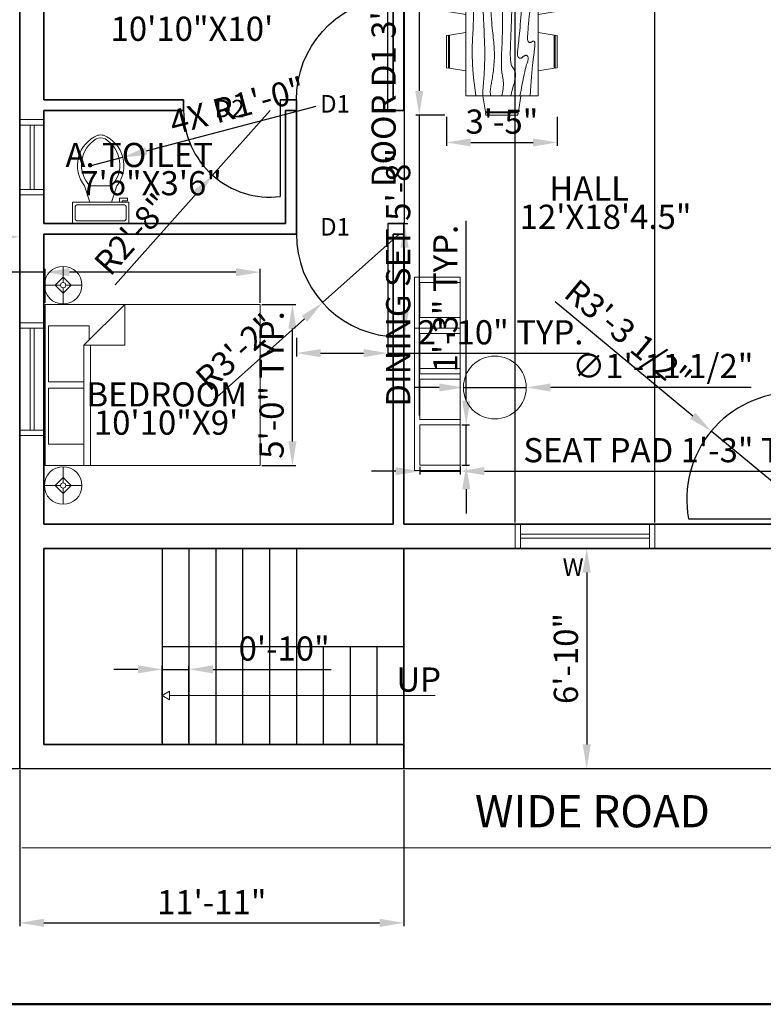
# Model space of a CAD drawing. Units: inches. Extents: x 2113 to 4530, y 1685 to 2353.
# Tile 2 of 6: x 2314 to 2591, y 1685 to 2052. Entities that reach past the tile are written whole.
import ezdxf

# ---------------------------------------------------------------- set-up
doc = ezdxf.new("R2010")
doc.units = ezdxf.units.IN
for name, color, linetype, lineweight in [('A-ANNO-DIMS', 2, 'Continuous', 18), ('A-ANNO-SYMB', 7, 'Continuous', 18), ('A-ANNO-TEXT', 7, 'Continuous', 18), ('A-ANNO-TTLB', 7, 'Continuous', 50), ('A-AREA-IDEN', 7, 'Continuous', 18), ('A-DOOR', 3, 'Continuous', 25), ('A-FLOR-FIXT', 9, 'Continuous', 18), ('A-FLOR-STRS', 7, 'Continuous', 25), ('A-FURN', 8, 'Continuous', 18), ('A-GLAZ', 4, 'Continuous', 18), ('A-WALL', 7, 'Continuous', 35), ('C-PROP', 7, 'Continuous', 25), ('C-ROAD', 8, 'Continuous', 18), ('S-ANNO-DIMS', 2, 'Continuous', 18)]:
    doc.layers.add(name, color=color, linetype=linetype, lineweight=lineweight)
doc.styles.get("Standard").update_dxf_attribs({"font": 'arial.ttf'})
doc.dimstyles.new('ISO-25', dxfattribs={"dimtxt": 9, "dimasz": 9, "dimexe": 1.25, "dimexo": 0.625, "dimgap": 2, "dimtad": 1, "dimdec": 1, "dimlunit": 4, "dimtxsty": 'Standard', "dimcen": 2.5, "dimazin": 0, "dimtfac": 1, "dimtdec": 1, "dimtmove": 0, "dimatfit": 3, "dimfxl": 1, "dimarcsym": 0})

# ---------------------------------------------------------------- blocks, each defined once
blk = doc.blocks.new('Toilet - top')
for p, q in [((9.5, -6), (9.5, -2)), ((-10, -8.5), (-8, -8.5)), ((-10, -9.5), (-10, -8.5)), ((-7, -9.5), (-10, -9.5)), ((-8, -8.5), (-8, -8)), ((-7, -8), (-7, -9.5)), ((-4, -8), (-6, -14)), ((4, -8), (6, -14)), ((4, -14), (-4, -14))]:
    blk.add_line(p, q)
blk.add_lwpolyline([(10.5, -8), (10.5, 0), (-10.5, 0), (-10.5, -8)], close=True)
for points in [[(-9.5, -2), (-9.5, -6)], [(8.5, -1), (-8.5, -1)], [(-8.5, -7), (8.5, -7)]]:
    blk.add_lwpolyline(points)
for centre, radius, start, end in [((-8.62, -1.88), 0.884, 81.8699, 188.1301), ((8.62, -1.88), 0.884, 351.8699, 98.1301), ((-8.62, -6.12), 0.884, 171.8699, 278.1301), ((8.62, -6.12), 0.884, 261.8699, 8.1301), ((3.52, -21.58), 12.17, 141.4691, 247.9714), ((4.2, -21.82), 11.33, 136.3677, 238.9468), ((-3.52, -21.58), 12.17, 292.0284, 38.5307), ((-4.2, -21.82), 11.33, 301.053, 43.6321), ((0, -27.88), 4, 245.7318, 294.2682), ((0, -29), 4, 254.8605, 285.1395)]:
    blk.add_arc(centre, radius, start, end)
blk = doc.blocks.new('Dining Set - 36 x 72 in.')
for p, q in [((-22.2343, 26.00059), (-23.4847, 17.99762)), ((-22.2304, 26), (-5.7608, 26)), ((-22, 27.5), (-22.1562, 26.50042)), ((-5.8416, 26.5), (-22.1534, 26.5)), ((-22, 27.5), (-6, 27.5)), ((-5.8437, 26.49966), (-6, 27.5)), ((-4.5152, 17.99762), (-5.7655, 25.99926)), ((5.7657, 26.00059), (4.5153, 17.99762)), ((5.7696, 26), (22.2392, 26)), ((6, 27.5), (5.8438, 26.50042)), ((22.1584, 26.5), (5.8466, 26.5)), ((6, 27.5), (22, 27.5)), ((22.1563, 26.49966), (22, 27.5)), ((23.4848, 17.99762), (22.2345, 25.99926)), ((36, 18), (-36, 18)), ((-36, 18), (-36, -18)), ((36, -18), (36, 18)), ((-45.5, 8), (-44.5004, 8.15617)), ((-45.5, 8), (-45.5, -8)), ((-44.5, -8.15843), (-44.5, 8.15338)), ((-44.0006, 8.23428), (-35.9976, 9.48474)), ((-44, 8.23041), (-44, -8.23915)), ((44.0006, 8.23428), (35.9976, 9.48474)), ((44, 8.23041), (44, -8.23915)), ((44.5, -8.15843), (44.5, 8.15338)), ((45.5, 8), (44.5005, 8.15617)), ((45.5, 8), (45.5, -8)), ((-44.4997, -8.15631), (-45.5, -8)), ((-35.9976, -9.48476), (-43.9993, -8.2345)), ((35.9976, -9.48476), (43.9993, -8.2345)), ((44.4997, -8.15631), (45.5, -8)), ((-36, -18), (36, -18)), ((-22.2343, -26.0006), (-23.4847, -17.99762)), ((-4.5152, -17.99762), (-5.7655, -25.99928)), ((5.7657, -26.0006), (4.5153, -17.99762)), ((23.4848, -17.99762), (22.2345, -25.99928)), ((-22.2304, -26), (-5.7608, -26)), ((-22, -27.5), (-22.1562, -26.50044)), ((-5.8416, -26.5), (-22.1534, -26.5)), ((-22, -27.5), (-6, -27.5)), ((-5.8437, -26.49967), (-6, -27.5)), ((5.7696, -26), (22.2392, -26)), ((6, -27.5), (5.8438, -26.50044)), ((22.1584, -26.5), (5.8466, -26.5)), ((6, -27.5), (22, -27.5)), ((22.1563, -26.49967), (22, -27.5))]:
    blk.add_line(p, q)
for points in [[(-36, 15), (-31.1772, 14.97754), (-26.8079, 14.91406), (-22.8538, 14.81543), (-19.276, 14.6875), (-16.0362, 14.53613), (-13.0957, 14.36718), (-10.4159, 14.18652), (-7.9583, 14), (-5.6904, 13.81315), (-3.6035, 13.63021), (-1.6954, 13.45508), (0.0365, 13.29166), (1.5945, 13.14388), (2.9811, 13.01562), (4.1988, 12.9108), (5.25, 12.83333), (6.1393, 12.78613), (6.8802, 12.76823), (7.4883, 12.77767), (7.9792, 12.8125), (8.3685, 12.87077), (8.6719, 12.95052), (8.9049, 13.0498), (9.0833, 13.16666), (9.2205, 13.29899), (9.3216, 13.44401), (9.3895, 13.59879), (9.4271, 13.76041), (9.4373, 13.92594), (9.4232, 14.09245), (9.3875, 14.257), (9.3333, 14.41666), (9.2638, 14.56917), (9.1836, 14.71484), (9.0975, 14.85465), (9.0104, 14.98958), (8.9272, 15.1206), (8.8529, 15.2487), (8.7922, 15.37483), (8.75, 15.5), (8.7305, 15.62467), (8.7344, 15.74739), (8.7617, 15.86621), (8.8125, 15.97916), (8.8867, 16.08431), (8.9844, 16.17968), (9.1055, 16.26334), (9.25, 16.33333), (9.4189, 16.38802), (9.6172, 16.42708), (9.8506, 16.45052), (10.125, 16.45833), (10.4463, 16.45052), (10.8203, 16.42708), (11.2529, 16.38802), (11.75, 16.33333), (12.3184, 16.26318), (12.9694, 16.17838), (13.7151, 16.07991), (14.5677, 15.96875), (15.5395, 15.84586), (16.6426, 15.71224), (17.8893, 15.56884), (19.2917, 15.41666), (20.859, 15.25667), (22.5879, 15.08984), (24.4721, 14.91715), (26.5052, 14.73958), (28.6809, 14.5581), (30.9929, 14.3737), (33.4347, 14.18733), (36, 14)], [(-36, 10), (-28.9766, 10.14274), (-23.1725, 10.20442), (-18.4241, 10.19775), (-14.5677, 10.13541), (-11.4399, 10.03011), (-8.877, 9.89453), (-6.7154, 9.74137), (-4.7917, 9.58333), (-2.9698, 9.43082), (-1.2246, 9.28515), (0.4415, 9.14534), (2.026, 9.01041), (3.5266, 8.87939), (4.9408, 8.7513), (6.266, 8.62516), (7.5, 8.5), (8.6411, 8.37549), (9.6914, 8.2539), (10.6538, 8.13818), (11.5312, 8.03125), (12.3267, 7.93603), (13.043, 7.85547), (13.6831, 7.79248), (14.25, 7.75), (14.7471, 7.7303), (15.1797, 7.73307), (15.5537, 7.75732), (15.875, 7.80208), (16.1494, 7.86637), (16.3828, 7.94922), (16.5811, 8.04964), (16.75, 8.16666), (16.8944, 8.29915), (17.0143, 8.44531), (17.1089, 8.60319), (17.1771, 8.77083), (17.218, 8.94629), (17.2305, 9.1276), (17.2137, 9.31282), (17.1667, 9.5), (17.0895, 9.6875), (16.987, 9.875), (16.8649, 10.0625), (16.7292, 10.25), (16.5856, 10.4375), (16.4401, 10.625), (16.2985, 10.8125), (16.1667, 11), (16.05, 11.18733), (15.9518, 11.3737), (15.8752, 11.5581), (15.8229, 11.73958), (15.798, 11.91715), (15.8034, 12.08984), (15.842, 12.25667), (15.9167, 12.41666), (16.0295, 12.56836), (16.1784, 12.70833), (16.3605, 12.83268), (16.5729, 12.9375), (16.8127, 13.01888), (17.0768, 13.07291), (17.3625, 13.0957), (17.6667, 13.08333), (17.9894, 13.03312), (18.3418, 12.94726), (18.7382, 12.82918), (19.1927, 12.68229), (19.7195, 12.51001), (20.3327, 12.31575), (21.0465, 12.10294), (21.875, 11.875), (22.8357, 11.63354), (23.959, 11.37304), (25.2786, 11.08618), (26.8282, 10.76562), (28.6414, 10.40405), (30.752, 9.99414), (33.1936, 9.52856), (36, 9)], [(-36, 5.5), (-30.7157, 5.3348), (-26.069, 5.20963), (-21.9946, 5.11767), (-18.4271, 5.05208), (-15.3009, 5.00602), (-12.5508, 4.97265), (-10.1112, 4.94515), (-7.9167, 4.91666), (-5.909, 4.88167), (-4.0586, 4.83984), (-2.3429, 4.79215), (-0.7396, 4.73958), (0.7739, 4.6831), (2.22, 4.6237), (3.6213, 4.56233), (5, 4.5), (6.373, 4.43782), (7.7344, 4.3776), (9.0723, 4.32129), (10.375, 4.27083), (11.6309, 4.22819), (12.8281, 4.19531), (13.9551, 4.17415), (15, 4.16666), (15.954, 4.17448), (16.819, 4.19791), (17.6001, 4.23698), (18.3021, 4.29166), (18.9299, 4.36198), (19.4883, 4.44791), (19.9823, 4.54948), (20.4167, 4.66666), (20.7969, 4.79899), (21.1302, 4.94401), (21.4245, 5.09879), (21.6875, 5.26041), (21.9271, 5.42594), (22.1511, 5.59245), (22.3672, 5.757), (22.5834, 5.91666), (22.8065, 6.06868), (23.0404, 6.21093), (23.2879, 6.34147), (23.5521, 6.45833), (23.8358, 6.55957), (24.142, 6.64323), (24.4735, 6.70735), (24.8334, 6.75), (25.2235, 6.76969), (25.642, 6.76692), (26.0858, 6.74267), (26.5521, 6.69791), (27.0379, 6.63362), (27.5404, 6.55078), (28.0565, 6.45036), (28.5834, 6.33333), (29.1242, 6.19987), (29.7071, 6.04687), (30.3661, 5.87044), (31.1354, 5.66666), (32.0493, 5.43164), (33.142, 5.16146), (34.4475, 4.85221), (36, 4.5)], [(-36, -1), (-30.7915, -0.6591), (-26.0195, -0.38216), (-21.6519, -0.16284), (-17.6563, 0.00521), (-14.0005, 0.12833), (-10.6523, 0.21289), (-7.5796, 0.26522), (-4.75, 0.29166), (-2.134, 0.29793), (0.2878, 0.28711), (2.5317, 0.26163), (4.6146, 0.22396), (6.5529, 0.17651), (8.3633, 0.12174), (10.0623, 0.06209), (11.6667, 0), (13.1899, -0.06201), (14.6341, -0.1211), (15.9982, -0.17432), (17.2813, -0.21875), (18.4823, -0.25147), (19.6003, -0.26953), (20.6343, -0.27002), (21.5834, -0.25), (22.4481, -0.20768), (23.2357, -0.14584), (23.9549, -0.06836), (24.6146, 0.02083), (25.2235, 0.11784), (25.7904, 0.21875), (26.3241, 0.31966), (26.8334, 0.41666), (27.3265, 0.50618), (27.8099, 0.58593), (28.2894, 0.65397), (28.7709, 0.70833), (29.2601, 0.74707), (29.763, 0.76823), (30.2855, 0.76985), (30.8334, 0.75), (31.4088, 0.70784), (31.9994, 0.64713), (32.589, 0.57275), (33.1615, 0.48958), (33.7008, 0.4025), (34.1908, 0.3164), (34.6153, 0.23616), (34.9584, 0.16666), (35.2099, 0.11165), (35.3848, 0.07031), (35.504, 0.04069), (35.5886, 0.02083), (35.6594, 0.00879), (35.7377, 0.0026), (35.8442, 0.00032), (36, 0)], [(-36, -6.5), (-27.1843, -6.31267), (-20.084, -6.1263), (-14.469, -5.9419), (-10.1094, -5.76042), (-6.7752, -5.58285), (-4.2363, -5.41016), (-2.2629, -5.24333), (-0.625, -5.08334), (0.8708, -4.93099), (2.2715, -4.78646), (3.5872, -4.64974), (4.8281, -4.52084), (6.0046, -4.39974), (7.127, -4.28646), (8.2053, -4.18099), (9.25, -4.08334), (10.2705, -3.99382), (11.2734, -3.91407), (12.2647, -3.84603), (13.25, -3.79167), (14.2354, -3.75293), (15.2266, -3.73177), (16.2295, -3.73015), (17.25, -3.75), (18.2912, -3.79248), (19.3451, -3.85547), (20.4009, -3.93604), (21.4479, -4.03125), (22.4754, -4.13819), (23.4727, -4.25391), (24.4289, -4.37549), (25.3334, -4.5), (26.1785, -4.62492), (26.9694, -4.74935), (27.7145, -4.87281), (28.4219, -4.99479), (29.1, -5.11483), (29.7572, -5.23242), (30.4016, -5.34709), (31.0417, -5.45834), (31.6837, -5.56437), (32.3262, -5.65821), (32.9658, -5.73153), (33.599, -5.77604), (34.2224, -5.78345), (34.8327, -5.74545), (35.4264, -5.65373), (36, -5.5)], [(-36, -10), (-26.4022, -9.81299), (-18.4675, -9.62891), (-11.9839, -9.45069), (-6.7396, -9.28125), (-2.5226, -9.12354), (0.8789, -8.98047), (3.6769, -8.85498), (6.0833, -8.75), (8.2767, -8.66765), (10.3021, -8.60677), (12.1712, -8.56543), (13.8958, -8.54167), (15.4876, -8.53353), (16.9583, -8.53907), (18.3197, -8.55632), (19.5834, -8.58334), (20.7616, -8.61841), (21.8685, -8.66081), (22.9188, -8.71004), (23.9271, -8.76563), (24.9081, -8.82707), (25.8763, -8.89388), (26.8465, -8.96558), (27.8334, -9.04167), (28.8474, -9.12118), (29.8828, -9.20117), (30.93, -9.27824), (31.9792, -9.34896), (33.0205, -9.40991), (34.0443, -9.45768), (35.0407, -9.48885), (36, -9.5)], [(-36, -14.5), (-30.0881, -14.33513), (-25.0332, -14.21224), (-20.7312, -14.12647), (-17.0781, -14.07292), (-13.97, -14.04671), (-11.3027, -14.04297), (-8.9724, -14.05681), (-6.875, -14.08334), (-4.9224, -14.11833), (-3.0905, -14.16016), (-1.3709, -14.20785), (0.2448, -14.26042), (1.7647, -14.3169), (3.1973, -14.3763), (4.5507, -14.43767), (5.8333, -14.5), (7.0554, -14.5621), (8.235, -14.62175), (9.3922, -14.67652), (10.5469, -14.72396), (11.7192, -14.76164), (12.929, -14.78711), (14.1965, -14.79794), (15.5417, -14.79167), (16.9933, -14.76424), (18.6152, -14.70508), (20.4804, -14.60197), (22.6615, -14.44271), (25.2312, -14.21509), (28.2624, -13.9069), (31.8277, -13.50594), (36, -13)]]:
    blk.add_lwpolyline(points)
blk = doc.blocks.new('Bed - Queen')
for p, q in [((0, -80.00003), (0, 0)), ((0, 0), (59.99999, 0)), ((59.99999, 0), (59.99999, -80.00003)), ((7.99999, -1.2), (28.79998, -1.2)), ((7.99999, -14.4), (7.99999, -1.2)), ((28.79998, -1.2), (28.79998, -14.4)), ((31.19999, -1.2), (51.99999, -1.2)), ((31.19999, -14.4), (31.19999, -1.2)), ((51.99999, -1.2), (51.99999, -16.4)), ((0, -14.4), (44.8, -14.4)), ((59.99999, -29.6), (44.8, -14.4)), ((44.8, -14.4), (44.8, -29.6)), ((44.8, -16.8), (0, -16.8)), ((51.99999, -16.4), (46.79936, -16.4)), ((44.8, -29.6), (59.99999, -29.6)), ((59.99999, -80.00003), (0, -80.00003))]:
    blk.add_line(p, q)
blk = doc.blocks.new('Lamp - Table')
for p, q in [((0, 7), (0, 1)), ((-1, 0), (-7, 0)), ((0, 3), (-3, 0)), ((-3, 0), (0, -3)), ((3, 0), (0, 3)), ((0, -3), (3, 0)), ((1, 0), (7, 0)), ((0, -1), (0, -7))]:
    blk.add_line(p, q)
for radius in [7, 1]:
    blk.add_circle((0, 0), radius)
blk = doc.blocks.new('*D26')
at = {"layer": 'A-ANNO-DIMS', "color": 0, "lineweight": -2, "transparency": 16777216}
for p, q in [((2457.36, 1854.89), (2526.08, 1854.89)), ((2524.83, 1845.89), (2524.83, 1781.89)), ((2457.36, 1772.89), (2526.08, 1772.89))]:
    blk.add_line(p, q, dxfattribs=at)
at = {"layer": 'A-ANNO-DIMS', "color": 0, "transparency": 16777216}
for points in [[(2523.33, 1845.89), (2526.33, 1845.89), (2524.83, 1854.89)], [(2523.33, 1781.89), (2526.33, 1781.89), (2524.83, 1772.89)]]:
    blk.add_solid(points, dxfattribs=at)
at = {"layer": 'Defpoints', "color": 0, "transparency": 16777216}
for p in [(2456.73, 1854.89), (2456.73, 1772.89), (2524.83, 1772.89)]:
    blk.add_point(p, dxfattribs=at)
at = {"layer": 'A-ANNO-DIMS', "color": 0, "transparency": 16777216, "insert": (2518.23, 1813.89), "char_height": 9, "attachment_point": 5, "rotation": 90}
blk.add_mtext('6\'-10"', dxfattribs=at)
blk = doc.blocks.new('*D29')
at = {"layer": 'A-ANNO-DIMS', "color": 0, "lineweight": -2, "transparency": 16777216}
for p, q in [((2289.73, 2168.26), (2289.73, 1969.64)), ((2313.73, 2150.26), (2313.73, 1969.64)), ((2304.73, 1970.89), (2298.73, 1970.89))]:
    blk.add_line(p, q, dxfattribs=at)
at = {"layer": 'A-ANNO-DIMS', "color": 0, "transparency": 16777216}
for points in [[(2298.73, 1972.39), (2298.73, 1969.39), (2289.73, 1970.89)], [(2304.73, 1972.39), (2304.73, 1969.39), (2313.73, 1970.89)]]:
    blk.add_solid(points, dxfattribs=at)
at = {"layer": 'Defpoints', "color": 0, "transparency": 16777216}
for p in [(2289.73, 2168.89), (2313.73, 2150.89), (2289.73, 1970.89)]:
    blk.add_point(p, dxfattribs=at)
at = {"layer": 'A-ANNO-DIMS', "color": 0, "transparency": 16777216, "insert": (2301.73, 1977.4), "char_height": 9, "attachment_point": 5}
blk.add_mtext("2'", dxfattribs=at)
blk = doc.blocks.new('DOOR-D1-SWING')
blk.add_line((34, 42), (34, 0))
blk.add_arc((38.24, 38), 38.24, 180, 263.6403)
blk = doc.blocks.new('SOFA-SEAT-PAD')
for p, q in [((0, 15), (0, 0)), ((0, 15), (15, 15)), ((0, 0), (15, 0))]:
    blk.add_line(p, q)
blk = doc.blocks.new('LOT-465X396')
blk.add_line((0, 0), (465, 0))
blk = doc.blocks.new('*D40')
at = {"layer": 'Defpoints', "color": 0, "transparency": 16777216}
for p in [(2323.25, 1957.72), (2323.25, 1945.72), (2403.25, 1945.72)]:
    blk.add_point(p, dxfattribs=at)
at = {"layer": 'S-ANNO-DIMS', "color": 0, "lineweight": -2, "transparency": 16777216}
for p, q in [((2323.25, 1946.35), (2323.25, 1958.97)), ((2403.25, 1946.35), (2403.25, 1958.97)), ((2323.25, 1957.72), (2177.86, 1957.72)), ((2394.25, 1957.72), (2332.25, 1957.72))]:
    blk.add_line(p, q, dxfattribs=at)
at = {"layer": 'S-ANNO-DIMS', "color": 0, "transparency": 16777216}
for points in [[(2332.25, 1959.22), (2332.25, 1956.22), (2323.25, 1957.72)], [(2394.25, 1959.22), (2394.25, 1956.22), (2403.25, 1957.72)]]:
    blk.add_solid(points, dxfattribs=at)
at = {"layer": 'S-ANNO-DIMS', "color": 0, "transparency": 16777216, "insert": (2246.05, 1964.65), "char_height": 9, "attachment_point": 5}
blk.add_mtext('QUEEN BED 6\'-8" TYP.', dxfattribs=at)
blk = doc.blocks.new('*D41')
at = {"layer": 'Defpoints', "color": 0, "transparency": 16777216}
for p in [(2403.25, 1945.72), (2415.25, 1945.72), (2403.25, 1885.72)]:
    blk.add_point(p, dxfattribs=at)
at = {"layer": 'S-ANNO-DIMS', "color": 0, "lineweight": -2, "transparency": 16777216}
for p, q in [((2403.87, 1945.72), (2416.5, 1945.72)), ((2415.25, 1894.72), (2415.25, 1936.72)), ((2403.87, 1885.72), (2416.5, 1885.72))]:
    blk.add_line(p, q, dxfattribs=at)
at = {"layer": 'S-ANNO-DIMS', "color": 0, "transparency": 16777216}
for points in [[(2413.75, 1936.72), (2416.75, 1936.72), (2415.25, 1945.72)], [(2413.75, 1894.72), (2416.75, 1894.72), (2415.25, 1885.72)]]:
    blk.add_solid(points, dxfattribs=at)
at = {"layer": 'S-ANNO-DIMS', "color": 0, "transparency": 16777216, "insert": (2408.65, 1915.72), "char_height": 9, "attachment_point": 5, "rotation": 90}
blk.add_mtext('5\'-0" TYP.', dxfattribs=at)
blk = doc.blocks.new('*D50')
at = {"layer": 'Defpoints', "color": 0, "transparency": 16777216}
for p in [(2462.73, 1885.89), (2477.73, 1885.89), (2477.73, 1883.64)]:
    blk.add_point(p, dxfattribs=at)
at = {"layer": 'S-ANNO-DIMS', "color": 0, "lineweight": -2, "transparency": 16777216}
for p, q in [((2462.73, 1885.26), (2462.73, 1882.39)), ((2477.73, 1885.26), (2477.73, 1882.39)), ((2453.73, 1883.64), (2444.73, 1883.64)), ((2462.73, 1883.64), (2477.73, 1883.64)), ((2486.73, 1883.64), (2620.23, 1883.64))]:
    blk.add_line(p, q, dxfattribs=at)
at = {"layer": 'S-ANNO-DIMS', "color": 0, "transparency": 16777216}
for points in [[(2453.73, 1885.14), (2453.73, 1882.14), (2462.73, 1883.64)], [(2486.73, 1885.14), (2486.73, 1882.14), (2477.73, 1883.64)]]:
    blk.add_solid(points, dxfattribs=at)
at = {"layer": 'S-ANNO-DIMS', "color": 0, "transparency": 16777216, "insert": (2557.98, 1890.29), "char_height": 9, "attachment_point": 5}
blk.add_mtext('SEAT PAD 1\'-3" TYP.', dxfattribs=at)
blk = doc.blocks.new('*D51')
at = {"layer": 'Defpoints', "color": 0, "transparency": 16777216}
for p in [(2477.73, 1900.89), (2479.98, 1900.89), (2477.73, 1885.89)]:
    blk.add_point(p, dxfattribs=at)
at = {"layer": 'S-ANNO-DIMS', "color": 0, "lineweight": -2, "transparency": 16777216}
for p, q in [((2479.98, 1909.89), (2479.98, 1976.9)), ((2478.36, 1900.89), (2481.23, 1900.89)), ((2479.98, 1885.89), (2479.98, 1900.89)), ((2478.36, 1885.89), (2481.23, 1885.89)), ((2479.98, 1876.89), (2479.98, 1867.89))]:
    blk.add_line(p, q, dxfattribs=at)
at = {"layer": 'S-ANNO-DIMS', "color": 0, "transparency": 16777216}
for points in [[(2478.48, 1909.89), (2481.48, 1909.89), (2479.98, 1900.89)], [(2478.48, 1876.89), (2481.48, 1876.89), (2479.98, 1885.89)]]:
    blk.add_solid(points, dxfattribs=at)
at = {"layer": 'S-ANNO-DIMS', "color": 0, "transparency": 16777216, "insert": (2473.38, 1947.89), "char_height": 9, "attachment_point": 5, "rotation": 90}
blk.add_mtext('1\'-3" TYP.', dxfattribs=at)
blk = doc.blocks.new('*D54')
at = {"layer": 'Defpoints', "color": 0, "transparency": 16777216}
for p in [(2450.73, 1975.89), (2457.03, 1975.89), (2450.73, 1933.89)]:
    blk.add_point(p, dxfattribs=at)
at = {"layer": 'S-ANNO-DIMS', "color": 0, "lineweight": -2, "transparency": 16777216}
for p, q in [((2457.03, 1975.89), (2457.03, 2104.07)), ((2451.36, 1975.89), (2458.28, 1975.89)), ((2457.03, 1942.89), (2457.03, 1966.89)), ((2451.36, 1933.89), (2458.28, 1933.89))]:
    blk.add_line(p, q, dxfattribs=at)
at = {"layer": 'S-ANNO-DIMS', "color": 0, "transparency": 16777216}
for points in [[(2455.53, 1966.89), (2458.53, 1966.89), (2457.03, 1975.89)], [(2455.53, 1942.89), (2458.53, 1942.89), (2457.03, 1933.89)]]:
    blk.add_solid(points, dxfattribs=at)
at = {"layer": 'S-ANNO-DIMS', "color": 0, "transparency": 16777216, "insert": (2450.37, 2044.48), "char_height": 9, "attachment_point": 5, "rotation": 90}
blk.add_mtext('DOOR D1 3\'-6" TYP.', dxfattribs=at)
blk = doc.blocks.new('*D55')
at = {"layer": 'Defpoints', "color": 0, "transparency": 16777216}
for p in [(2416.73, 1933.89), (2450.73, 1933.89), (2450.73, 1927.59)]:
    blk.add_point(p, dxfattribs=at)
at = {"layer": 'S-ANNO-DIMS', "color": 0, "lineweight": -2, "transparency": 16777216}
for p, q in [((2416.73, 1933.26), (2416.73, 1926.34)), ((2450.73, 1933.26), (2450.73, 1926.34)), ((2425.73, 1927.59), (2441.73, 1927.59)), ((2450.73, 1927.59), (2525.74, 1927.59))]:
    blk.add_line(p, q, dxfattribs=at)
at = {"layer": 'S-ANNO-DIMS', "color": 0, "transparency": 16777216}
for points in [[(2425.73, 1929.09), (2425.73, 1926.09), (2416.73, 1927.59)], [(2441.73, 1929.09), (2441.73, 1926.09), (2450.73, 1927.59)]]:
    blk.add_solid(points, dxfattribs=at)
at = {"layer": 'S-ANNO-DIMS', "color": 0, "transparency": 16777216, "insert": (2492.74, 1934.18), "char_height": 9, "attachment_point": 5}
blk.add_mtext('2\'-10" TYP.', dxfattribs=at)
blk = doc.blocks.new('*D58')
at = {"layer": 'Defpoints', "color": 0, "transparency": 16777216}
for p in [(2472.67, 2084.34), (2462.46, 2016.25), (2472.67, 2016.25)]:
    blk.add_point(p, dxfattribs=at)
at = {"layer": 'S-ANNO-DIMS', "color": 0, "lineweight": -2, "transparency": 16777216}
for p, q in [((2472.05, 2084.34), (2461.21, 2084.34)), ((2462.46, 2075.34), (2462.46, 2025.25)), ((2472.05, 2016.25), (2461.21, 2016.25)), ((2462.46, 2016.25), (2462.46, 1904.33))]:
    blk.add_line(p, q, dxfattribs=at)
at = {"layer": 'S-ANNO-DIMS', "color": 0, "transparency": 16777216}
for points in [[(2460.96, 2075.34), (2463.96, 2075.34), (2462.46, 2084.34)], [(2460.96, 2025.25), (2463.96, 2025.25), (2462.46, 2016.25)]]:
    blk.add_solid(points, dxfattribs=at)
at = {"layer": 'S-ANNO-DIMS', "color": 0, "transparency": 16777216, "insert": (2455.81, 1955.79), "char_height": 9, "attachment_point": 5, "rotation": 90}
blk.add_mtext('DINING SET 5\'-8"', dxfattribs=at)
blk = doc.blocks.new('*D59')
at = {"layer": 'Defpoints', "color": 0, "transparency": 16777216}
for p in [(2472.67, 2016.25), (2513.83, 2016.25), (2513.83, 2006.03)]:
    blk.add_point(p, dxfattribs=at)
at = {"layer": 'S-ANNO-DIMS', "color": 0, "lineweight": -2, "transparency": 16777216}
for p, q in [((2472.67, 2015.62), (2472.67, 2004.78)), ((2513.83, 2015.62), (2513.83, 2004.78)), ((2481.67, 2006.03), (2504.83, 2006.03))]:
    blk.add_line(p, q, dxfattribs=at)
at = {"layer": 'S-ANNO-DIMS', "color": 0, "transparency": 16777216}
for points in [[(2481.67, 2007.53), (2481.67, 2004.53), (2472.67, 2006.03)], [(2504.83, 2007.53), (2504.83, 2004.53), (2513.83, 2006.03)]]:
    blk.add_solid(points, dxfattribs=at)
at = {"layer": 'S-ANNO-DIMS', "color": 0, "transparency": 16777216, "insert": (2493.25, 2012.63), "char_height": 9, "attachment_point": 5}
blk.add_mtext('3\'-5"', dxfattribs=at)
blk = doc.blocks.new('*D90')
at = {"layer": 'Defpoints', "color": 0, "transparency": 16777216}
for p in [(2313.73, 1772.89), (2456.73, 1772.89), (2456.73, 1715.45)]:
    blk.add_point(p, dxfattribs=at)
at = {"layer": 'S-ANNO-DIMS', "color": 0, "lineweight": -2, "transparency": 16777216}
for p, q in [((2313.73, 1772.26), (2313.73, 1714.2)), ((2456.73, 1772.26), (2456.73, 1714.2)), ((2322.73, 1715.45), (2447.73, 1715.45))]:
    blk.add_line(p, q, dxfattribs=at)
at = {"layer": 'S-ANNO-DIMS', "color": 0, "transparency": 16777216}
for points in [[(2322.73, 1716.95), (2322.73, 1713.95), (2313.73, 1715.45)], [(2447.73, 1716.95), (2447.73, 1713.95), (2456.73, 1715.45)]]:
    blk.add_solid(points, dxfattribs=at)
at = {"layer": 'S-ANNO-DIMS', "color": 0, "transparency": 16777216, "insert": (2385.23, 1721.97), "char_height": 9, "attachment_point": 5}
blk.add_mtext('11\'-11"', dxfattribs=at)
blk = doc.blocks.new('*D93')
at = {"layer": 'Defpoints', "color": 0, "transparency": 16777216}
for p in [(2550.184017, 2196.835797), (2498.184017, 1863.885797), (2550.184017, 1863.885797)]:
    blk.add_point(p, dxfattribs=at)
at = {"layer": 'S-ANNO-DIMS', "color": 0, "lineweight": -2, "transparency": 16777216}
for p, q in [((2498.184017, 1864.510797), (2498.184017, 2198.085797)), ((2507.184017, 2196.835797), (2541.184017, 2196.835797)), ((2550.184017, 1864.510797), (2550.184017, 2198.085797))]:
    blk.add_line(p, q, dxfattribs=at)
at = {"layer": 'S-ANNO-DIMS', "color": 0, "transparency": 16777216}
for points in [[(2507.184017, 2198.335797), (2507.184017, 2195.335797), (2498.184017, 2196.835797)], [(2541.184017, 2198.335797), (2541.184017, 2195.335797), (2550.184017, 2196.835797)]]:
    blk.add_solid(points, dxfattribs=at)
at = {"layer": 'S-ANNO-DIMS', "color": 0, "transparency": 16777216, "insert": (2524.184017, 2203.335797), "char_height": 9, "attachment_point": 5}
blk.add_mtext('4\'-4"', dxfattribs=at)
blk = doc.blocks.new('*D94')
at = {"layer": 'Defpoints', "color": 0, "transparency": 16777216}
for p in [(2376.73, 1809.84), (2366.73, 1781.89), (2376.73, 1781.89)]:
    blk.add_point(p, dxfattribs=at)
at = {"layer": 'S-ANNO-DIMS', "color": 0, "lineweight": -2, "transparency": 16777216}
for p, q in [((2357.73, 1809.84), (2348.73, 1809.84)), ((2366.73, 1782.51), (2366.73, 1811.09)), ((2366.73, 1809.84), (2376.73, 1809.84)), ((2376.73, 1782.51), (2376.73, 1811.09)), ((2385.73, 1809.84), (2429.65, 1809.84))]:
    blk.add_line(p, q, dxfattribs=at)
at = {"layer": 'S-ANNO-DIMS', "color": 0, "transparency": 16777216}
for points in [[(2357.73, 1811.34), (2357.73, 1808.34), (2366.73, 1809.84)], [(2385.73, 1811.34), (2385.73, 1808.34), (2376.73, 1809.84)]]:
    blk.add_solid(points, dxfattribs=at)
at = {"layer": 'S-ANNO-DIMS', "color": 0, "transparency": 16777216, "insert": (2412.19, 1816.43), "char_height": 9, "attachment_point": 5}
blk.add_mtext('0\'-10"', dxfattribs=at)
blk = doc.blocks.new('*D102')
at = {"layer": 'Defpoints', "color": 0, "transparency": 16777216}
for p in [(2571.2, 1898.54), (2601.73, 1873.2)]:
    blk.add_point(p, dxfattribs=at)
at = {"layer": 'S-ANNO-DIMS', "color": 0, "lineweight": -2, "transparency": 16777216}
for p, q in [((2513.09, 1946.76), (2564.27, 1904.29)), ((2601.73, 1873.2), (2571.2, 1898.54))]:
    blk.add_line(p, q, dxfattribs=at)
at = {"layer": 'S-ANNO-DIMS', "color": 0, "transparency": 16777216}
blk.add_solid([(2565.23, 1905.45), (2563.31, 1903.14), (2571.2, 1898.54)], dxfattribs=at)
at = {"layer": 'S-ANNO-DIMS', "color": 0, "transparency": 16777216, "insert": (2539.47, 1933.52), "char_height": 9, "attachment_point": 5, "rotation": 320.315}
blk.add_mtext('R3\'-3 1/2"', dxfattribs=at)
blk = doc.blocks.new('*D104')
at = {"layer": 'Defpoints', "color": 0, "transparency": 16777216}
for p in [(2454.97, 1971.89), (2426.47, 1946.39)]:
    blk.add_point(p, dxfattribs=at)
at = {"layer": 'S-ANNO-DIMS', "color": 0, "lineweight": -2, "transparency": 16777216}
for p, q in [((2454.97, 1971.89), (2426.47, 1946.39)), ((2385.83, 1910.03), (2419.77, 1940.39))]:
    blk.add_line(p, q, dxfattribs=at)
at = {"layer": 'S-ANNO-DIMS', "color": 0, "transparency": 16777216}
blk.add_solid([(2418.77, 1941.51), (2420.77, 1939.27), (2426.47, 1946.39)], dxfattribs=at)
at = {"layer": 'S-ANNO-DIMS', "color": 0, "transparency": 16777216, "insert": (2395.04, 1927.12), "char_height": 9, "attachment_point": 5, "rotation": 41.8197}
blk.add_mtext('R3\'-2"', dxfattribs=at)
blk = doc.blocks.new('*D106')
at = {"layer": 'Defpoints', "color": 0, "transparency": 16777216}
for p in [(2406.95, 2017.89), (2385.55, 1993.8)]:
    blk.add_point(p, dxfattribs=at)
at = {"layer": 'S-ANNO-DIMS', "color": 0, "lineweight": -2, "transparency": 16777216}
for p, q in [((2406.95, 2017.89), (2385.55, 1993.8)), ((2349.31, 1953.04), (2379.57, 1987.08))]:
    blk.add_line(p, q, dxfattribs=at)
at = {"layer": 'S-ANNO-DIMS', "color": 0, "transparency": 16777216}
blk.add_solid([(2378.45, 1988.07), (2380.69, 1986.08), (2385.55, 1993.8)], dxfattribs=at)
at = {"layer": 'S-ANNO-DIMS', "color": 0, "transparency": 16777216, "insert": (2356.52, 1971.08), "char_height": 9, "attachment_point": 5, "rotation": 48.3656}
blk.add_mtext('R2\'-8"', dxfattribs=at)
blk = doc.blocks.new('*D107')
at = {"layer": 'Defpoints', "color": 0, "transparency": 16777216}
for p in [(2478.94, 1914.79), (2502.33, 1914.79)]:
    blk.add_point(p, dxfattribs=at)
at = {"layer": 'S-ANNO-DIMS', "color": 0, "lineweight": -2, "transparency": 16777216}
for p, q in [((2469.94, 1914.79), (2460.94, 1914.79)), ((2478.94, 1914.79), (2502.33, 1914.79)), ((2586.01, 1914.78), (2511.33, 1914.78))]:
    blk.add_line(p, q, dxfattribs=at)
at = {"layer": 'S-ANNO-DIMS', "color": 0, "transparency": 16777216}
for points in [[(2469.94, 1916.29), (2469.94, 1913.29), (2478.94, 1914.79)], [(2511.33, 1916.28), (2511.33, 1913.28), (2502.33, 1914.79)]]:
    blk.add_solid(points, dxfattribs=at)
at = {"layer": 'S-ANNO-DIMS', "color": 0, "transparency": 16777216, "insert": (2553.17, 1921.63), "char_height": 9, "attachment_point": 5, "rotation": 359.9989}
blk.add_mtext('∅1\'-11 1/2"', dxfattribs=at)
blk = doc.blocks.new('*D108')
at = {"layer": 'Defpoints', "color": 0, "transparency": 16777216}
for p in [(2352.13, 2000.5), (2340.36, 1997.41)]:
    blk.add_point(p, dxfattribs=at)
at = {"layer": 'S-ANNO-DIMS', "color": 0, "lineweight": -2, "transparency": 16777216}
for p, q in [((2423.93, 2019.36), (2360.84, 2002.79)), ((2340.36, 1997.41), (2352.13, 2000.5))]:
    blk.add_line(p, q, dxfattribs=at)
at = {"layer": 'S-ANNO-DIMS', "color": 0, "transparency": 16777216}
blk.add_solid([(2360.45, 2004.24), (2361.22, 2001.34), (2352.13, 2000.5)], dxfattribs=at)
at = {"layer": 'S-ANNO-DIMS', "color": 0, "transparency": 16777216, "insert": (2395.06, 2018.6), "char_height": 9, "attachment_point": 5, "rotation": 14.7198}
blk.add_mtext('4X R1\'-0"', dxfattribs=at)

msp = doc.modelspace()

# ---------------------------------------------------------------- linework, layer by layer
at = {"layer": 'A-ANNO-SYMB'}
for p, q in [((2366.73, 1800.14), (2369.51, 1801.73)), ((2366.73, 1800.14), (2369.51, 1798.54)), ((2369.51, 1801.73), (2369.51, 1798.54)), ((2369.51, 1800.14), (2468.39, 1800.14))]:
    msp.add_line(p, q, dxfattribs=at)
at = {"layer": 'A-ANNO-TTLB'}
msp.add_lwpolyline([(2112.77, 2352.97), (4498.42, 2352.97), (4498.42, 1685.12), (2112.77, 1685.12)], close=True, dxfattribs=at)
at = {"layer": 'A-DOOR'}
for p, q in [((2410.73, 2021.89), (2410.73, 1985.89)), ((2562.73, 1865.89), (2610.73, 1865.89))]:
    msp.add_line(p, q, dxfattribs=at)
for centre, radius, start, end in [((2406.95, 2017.89), 32.22, 180, 276.7329), ((2601.73, 1873.2), 39.68, 90, 190.6291)]:
    msp.add_arc(centre, radius, start, end, dxfattribs=at)
at = {"layer": 'A-FLOR-STRS'}
for p, q in [((2366.73, 1854.89), (2366.73, 1781.89)), ((2376.73, 1854.89), (2376.73, 1781.89)), ((2386.73, 1854.89), (2386.73, 1781.89)), ((2396.73, 1854.89), (2396.73, 1781.89)), ((2406.73, 1854.89), (2406.73, 1781.89)), ((2416.73, 1854.89), (2416.73, 1781.89)), ((2366.73, 1818.39), (2456.73, 1818.39)), ((2426.73, 1818.39), (2426.73, 1781.89)), ((2436.73, 1818.39), (2436.73, 1781.89)), ((2446.73, 1818.39), (2446.73, 1781.89))]:
    msp.add_line(p, q, dxfattribs=at)
at = {"layer": 'A-FURN'}
for p, q in [((2460.73, 1955.89), (2460.73, 1883.89)), ((2460.73, 1955.89), (2477.73, 1955.89)), ((2477.73, 1955.89), (2477.73, 1883.89)), ((2462.73, 1953.89), (2477.73, 1953.89)), ((2462.73, 1953.89), (2462.73, 1940.89)), ((2462.73, 1940.89), (2477.73, 1940.89)), ((2460.73, 1936.89), (2477.73, 1936.89)), ((2462.73, 1921.89), (2477.73, 1921.89)), ((2460.73, 1883.89), (2477.73, 1883.89))]:
    msp.add_line(p, q, dxfattribs=at)
msp.add_circle((2490.63, 1914.79), 11.69, dxfattribs=at)
at = {"layer": 'A-GLAZ'}
for p, q in [((2322.73, 2014.53), (2313.73, 2014.53)), ((2322.73, 2012.53), (2313.73, 2012.53)), ((2317.67, 1988.53), (2317.67, 2012.53)), ((2319.17, 1988.53), (2319.17, 2012.53)), ((2322.73, 1988.53), (2313.73, 1988.53)), ((2322.73, 1986.53), (2313.73, 1986.53)), ((2313.73, 1938.89), (2322.73, 1938.89)), ((2313.73, 1936.89), (2322.73, 1936.89)), ((2317.67, 1898.89), (2317.67, 1936.89)), ((2319.17, 1898.89), (2319.17, 1936.89)), ((2313.73, 1898.89), (2322.73, 1898.89)), ((2313.73, 1896.89), (2322.73, 1896.89)), ((2498.18, 1863.89), (2498.18, 1854.89)), ((2500.18, 1863.89), (2500.18, 1854.89)), ((2548.18, 1863.89), (2548.18, 1854.89)), ((2550.18, 1863.89), (2550.18, 1854.89)), ((2500.18, 1860.14), (2548.18, 1860.14)), ((2500.18, 1858.64), (2548.18, 1858.64))]:
    msp.add_line(p, q, dxfattribs=at)
at = {"layer": 'A-WALL'}
for p, q in [((2313.73, 2150.89), (2313.73, 1772.89)), ((2322.73, 2141.89), (2322.73, 2021.89)), ((2452.73, 2141.89), (2452.73, 2021.89)), ((2456.73, 2089.89), (2456.73, 2017.89)), ((2322.73, 2021.89), (2374.73, 2021.89)), ((2322.73, 2021.89), (2374.73, 2021.89)), ((2374.73, 2021.89), (2374.73, 2017.89)), ((2410.73, 2021.89), (2416.73, 2021.89)), ((2410.73, 2021.89), (2416.73, 2021.89)), ((2416.73, 2021.89), (2416.73, 1971.89)), ((2450.73, 2021.89), (2452.73, 2021.89)), ((2322.73, 2017.89), (2374.73, 2017.89)), ((2322.73, 2017.89), (2374.73, 2017.89)), ((2322.73, 2017.89), (2322.73, 1975.89)), ((2412.73, 2017.89), (2412.73, 1975.89)), ((2412.73, 2017.89), (2416.73, 2017.89)), ((2450.73, 2017.89), (2456.73, 2017.89)), ((2452.73, 2017.89), (2456.73, 2017.89)), ((2322.73, 1975.89), (2412.73, 1975.89)), ((2450.73, 1975.89), (2456.73, 1975.89)), ((2456.73, 1975.89), (2456.73, 1863.89)), ((2322.73, 1971.89), (2416.73, 1971.89)), ((2322.73, 1971.89), (2322.73, 1863.89)), ((2452.73, 1971.89), (2452.73, 1863.89)), ((2452.73, 1971.89), (2456.73, 1971.89)), ((2322.73, 1863.89), (2452.73, 1863.89)), ((2456.73, 1863.89), (2610.73, 1863.89)), ((2322.73, 1854.89), (2650.73, 1854.89)), ((2322.73, 1854.89), (2322.73, 1781.89)), ((2456.73, 1854.89), (2456.73, 1772.89)), ((2322.73, 1781.89), (2456.73, 1781.89))]:
    msp.add_line(p, q, dxfattribs=at)
at = {"layer": 'C-ROAD'}
msp.add_line((2314.56, 1743.4), (2754.73, 1743.4), dxfattribs=at)

# ---------------------------------------------------------------- block references
at = {"layer": 'A-DOOR', "extrusion": (0, 0, -1), "zscale": -1, "rotation": 180}
msp.add_blockref('DOOR-D1-SWING', (-2416.73, 2059.89), dxfattribs=at)
at = {"layer": 'A-DOOR'}
msp.add_blockref('DOOR-D1-SWING', (2416.73, 1933.89), dxfattribs=at)
at = {"layer": 'A-FLOR-FIXT', "rotation": 180}
msp.add_blockref('Toilet - top', (2343.88, 1975.83), dxfattribs=at)
at = {"layer": 'A-FURN', "xscale": 0.7483003964013882, "yscale": 0.7483003964013882, "zscale": 0.7483003964013882, "rotation": 269.9999999999999}
msp.add_blockref('Dining Set - 36 x 72 in.', (2493.25, 2050.3), dxfattribs=at)
at = {"layer": 'A-FURN'}
for name, p, rotation in [('Lamp - Table', (2329.91, 1952.9), 180), ('Bed - Queen', (2323.25, 1885.72), 90), ('Lamp - Table', (2329.91, 1878.29), 180)]:
    msp.add_blockref(name, p, dxfattribs=dict(at, rotation=rotation))
for p in [(2462.73, 1919.89), (2462.73, 1902.89), (2462.73, 1885.89)]:
    msp.add_blockref('SOFA-SEAT-PAD', p, dxfattribs=at)
at = {"layer": 'C-PROP'}
msp.add_blockref('LOT-465X396', (2289.73, 1772.89), dxfattribs=at)

# ---------------------------------------------------------------- texts
at = {"layer": 'A-ANNO-TEXT'}
for s, height, p in [(' D2', 6.54, (2384.32, 2015.36)), (' D1', 6.54, (2423.58, 2017.15)), (' D1', 6.54, (2423.58, 1971.35)), ('        W', 6.54, (2499.86, 1844.63)), ('    UP', 9, (2442.95, 1801.54)), ('    WIDE ROAD', 12, (2468.52, 1751.02))]:
    msp.add_text(s, height=height, dxfattribs=at).set_placement(p)
at = {"layer": 'A-AREA-IDEN'}
for s, p in [('   10\'10"X10\'', (2339.3, 2043.86)), ('A. TOILET', (2330.76, 1996.87)), ('  7\'6"X3\'6"', (2330.76, 1986.36)), ('       HALL', (2491.6, 1984.36)), ('   12\'X18\'4.5"', (2491.6, 1973.85)), ('  BEDROOM', (2333.09, 1907.72)), ('   10\'10"X9\'', (2333.09, 1897.21))]:
    msp.add_text(s, height=9, dxfattribs=at).set_placement(p)

# ---------------------------------------------------------------- dimensions: what is measured, and where the dimension line sits
at = {"layer": 'A-ANNO-DIMS'}
dim = msp.add_linear_dim(base=(2289.73, 1970.89), p1=(2313.73, 2150.89), p2=(2289.73, 2168.89), dimstyle='ISO-25', override={"dimclrd": 0, "dimclre": 0, "dimclrt": 0}, dxfattribs=at)
dim.commit()
dim.dimension.update_dxf_attribs({"geometry": '*D29', "text_midpoint": (2301.73, 1977.4)})
dim = msp.add_linear_dim(base=(2524.83, 1772.89), p1=(2456.73, 1854.89), p2=(2456.73, 1772.89), angle=90, dimstyle='ISO-25', override={"dimclrd": 0, "dimclre": 0, "dimclrt": 0}, dxfattribs=at)
dim.commit()
dim.dimension.update_dxf_attribs({"geometry": '*D26', "text_midpoint": (2518.23, 1813.89)})
at = {"layer": 'S-ANNO-DIMS'}
for base, p1, p2, picture, middle in [((2550.18, 2196.84), (2498.18, 1863.89), (2550.18, 1863.89), '*D93', (2524.18, 2203.34)), ((2513.83, 2006.03), (2472.67, 2016.25), (2513.83, 2016.25), '*D59', (2493.25, 2012.63)), ((2376.73, 1809.84), (2366.73, 1781.89), (2376.73, 1781.89), '*D94', (2412.19, 1816.43)), ((2456.73, 1715.45), (2313.73, 1772.89), (2456.73, 1772.89), '*D90', (2385.23, 1721.97))]:
    dim = msp.add_linear_dim(base=base, p1=p1, p2=p2, dimstyle='ISO-25', override={"dimdec": 1, "dimlfac": 1, "dimrnd": 0, "dimzin": 1, "dimdsep": 46, "dimlunit": 4, "dimfrac": 2}, dxfattribs=at)
    dim.commit()
    dim.dimension.update_dxf_attribs({"geometry": picture, "text_midpoint": middle})
for base, p1, p2, angle, text, picture, middle in [((2457.03, 1975.89), (2450.73, 1933.89), (2450.73, 1975.89), 90, 'DOOR D1 <> TYP.', '*D54', (2450.37, 2044.48)), ((2462.46, 2016.25), (2472.67, 2084.34), (2472.67, 2016.25), 270, 'DINING SET <>', '*D58', (2455.81, 1955.79)), ((2323.25, 1957.72), (2403.25, 1945.72), (2323.25, 1945.72), 180, 'QUEEN BED <> TYP.', '*D40', (2246.05, 1964.65)), ((2479.98, 1900.89), (2477.73, 1885.89), (2477.73, 1900.89), 90, '<> TYP.', '*D51', (2473.38, 1947.89)), ((2415.25, 1945.72), (2403.25, 1885.72), (2403.25, 1945.72), 90, '<> TYP.', '*D41', (2408.65, 1915.72))]:
    dim = msp.add_linear_dim(base=base, p1=p1, p2=p2, angle=angle, text=text, dimstyle='ISO-25', override={"dimdec": 1, "dimlfac": 1, "dimrnd": 0, "dimzin": 1, "dimdsep": 46, "dimlunit": 4, "dimfrac": 2}, dxfattribs=at)
    dim.commit()
    dim.dimension.update_dxf_attribs({"geometry": picture, "text_midpoint": middle})
dim = msp.add_radius_dim(center=(2340.36, 1997.41), mpoint=(2352.13, 2000.5), text='4X <>', dimstyle='ISO-25', override={"dimdec": 1, "dimlfac": 1, "dimrnd": 0, "dimzin": 1, "dimdsep": 46, "dimlunit": 4, "dimfrac": 2}, dxfattribs=at)
dim.commit()
dim.dimension.update_dxf_attribs({"geometry": '*D108', "text_midpoint": (2395.06, 2018.6)})
for center, mpoint, picture, middle in [((2406.95, 2017.89), (2385.55, 1993.8), '*D106', (2356.52, 1971.08)), ((2454.97, 1971.89), (2426.47, 1946.39), '*D104', (2395.04, 1927.12)), ((2601.73, 1873.2), (2571.2, 1898.54), '*D102', (2539.47, 1933.52))]:
    dim = msp.add_radius_dim(center=center, mpoint=mpoint, dimstyle='ISO-25', override={"dimdec": 1, "dimlfac": 1, "dimrnd": 0, "dimzin": 1, "dimdsep": 46, "dimlunit": 4, "dimfrac": 2}, dxfattribs=at)
    dim.commit()
    dim.dimension.update_dxf_attribs({"geometry": picture, "text_midpoint": middle})
for base, p1, p2, text, picture, middle in [((2450.73, 1927.59), (2416.73, 1933.89), (2450.73, 1933.89), '<> TYP.', '*D55', (2492.74, 1934.18)), ((2477.73, 1883.64), (2462.73, 1885.89), (2477.73, 1885.89), 'SEAT PAD <> TYP.', '*D50', (2557.98, 1890.29))]:
    dim = msp.add_linear_dim(base=base, p1=p1, p2=p2, text=text, dimstyle='ISO-25', override={"dimdec": 1, "dimlfac": 1, "dimrnd": 0, "dimzin": 1, "dimdsep": 46, "dimlunit": 4, "dimfrac": 2}, dxfattribs=at)
    dim.commit()
    dim.dimension.update_dxf_attribs({"geometry": picture, "text_midpoint": middle})
dim = msp.add_diameter_dim_2p(p1=(2478.94, 1914.79), p2=(2502.33, 1914.79), dimstyle='ISO-25', override={"dimdec": 1, "dimlfac": 1, "dimrnd": 0, "dimzin": 1, "dimdsep": 46, "dimlunit": 4, "dimfrac": 2}, dxfattribs=at)
dim.commit()
dim.dimension.update_dxf_attribs({"geometry": '*D107', "text_midpoint": (2553.17, 1914.78)})

doc.saveas('drawing.dxf')
